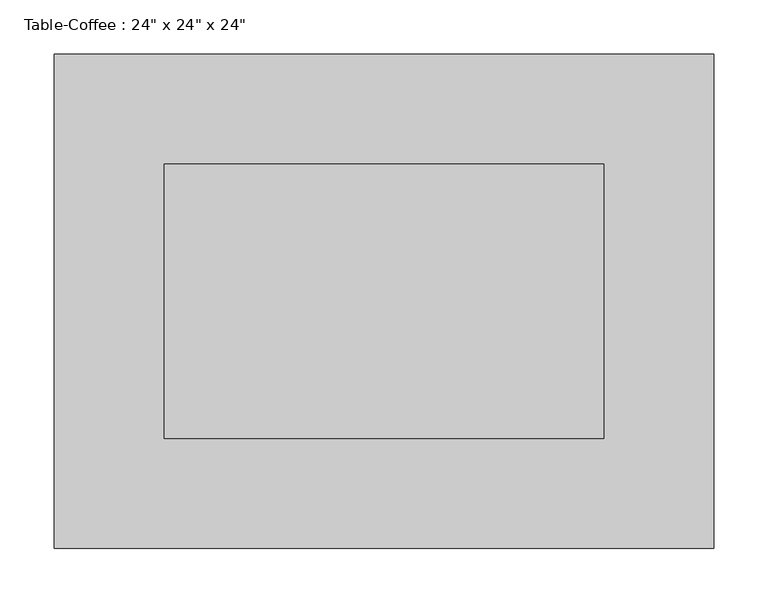
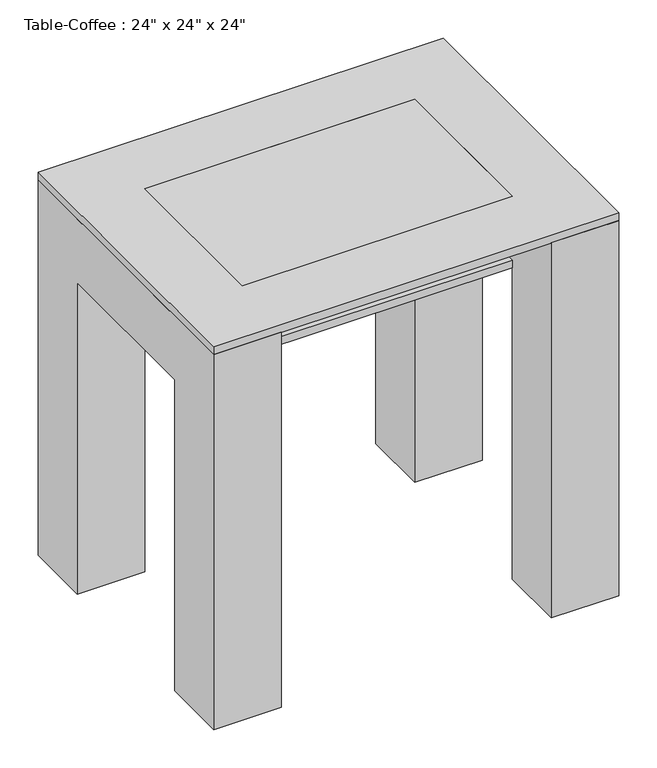
"""IFC4 building model written with IfcOpenShell, lengths in millimetres: furniture geometry."""

from ifc_helpers import new_model, si_unit, frame, origin, place, context, project, spatial, polyline, outline, extrude, source, transform, mapped, element, save


def furniture_7122704d(model_context):
    return source(origin(), model_context, "Body", "SweptSolid", [
        extrude(outline(polyline([(221.4657667, 222.2110778), (221.4657667, -31.7889222), (-184.9342333, -31.7889222), (-184.9342333, 222.2110778), (221.4657667, 222.2110778)])), frame((0.0, 0.0, 495.3), z_axis=(0.0, 0.0, 1.0), x_axis=(1.0, 0.0, 0.0)), (0.0, 0.0, 1.0), 12.7),
        extrude(outline(polyline([(323.8110778, 0.0), (222.2110778, 0.0), (222.2110778, 495.3), (-31.7889222, 495.3), (-31.7889222, 0.0), (-133.3889222, 0.0), (-133.3889222, 596.9), (323.8110778, 596.9), (323.8110778, 0.0)])), frame((221.4657667, 0.0, 0.0), z_axis=(1.0, 0.0, 0.0), x_axis=(0.0, 1.0, 0.0)), (0.0, 0.0, 1.0), 101.6),
        extrude(outline(polyline([(323.8110778, 596.9), (323.8110778, 0.0), (222.2110778, 0.0), (222.2110778, 495.3), (-31.7889222, 495.3), (-31.7889222, 0.0), (-133.3889222, 0.0), (-133.3889222, 596.9), (323.8110778, 596.9)])), frame((-286.5342333, 0.0, 0.0), z_axis=(1.0, 0.0, 0.0), x_axis=(0.0, 1.0, 0.0)), (0.0, 0.0, 1.0), 101.6),
        extrude(outline(polyline([(221.4657667, 222.2110778), (221.4657667, -31.7889222), (-184.9342333, -31.7889222), (-184.9342333, 222.2110778), (221.4657667, 222.2110778)])), frame((0.0, 0.0, 596.9), z_axis=(0.0, 0.0, 1.0), x_axis=(1.0, 0.0, 0.0)), (0.0, 0.0, 1.0), 12.7),
        extrude(outline(polyline([(323.0657667, 323.8110778), (323.0657667, -133.3889222), (-286.5342333, -133.3889222), (-286.5342333, 323.8110778), (323.0657667, 323.8110778)]), holes=[polyline([(221.4657667, 222.2110778), (-184.9342333, 222.2110778), (-184.9342333, -31.7889222), (221.4657667, -31.7889222), (221.4657667, 222.2110778)])]), frame((0.0, 0.0, 596.9), z_axis=(0.0, 0.0, 1.0), x_axis=(1.0, 0.0, 0.0)), (0.0, 0.0, 1.0), 12.7),
    ])


if __name__ == "__main__":
    model = new_model("IFC4")
    model_context = context("Model", 3, world=origin())
    ifc_project = project(units=[si_unit("LENGTHUNIT", "METRE", prefix="MILLI")], contexts=[model_context])
    site = spatial("IfcSite", under=ifc_project)
    building = spatial("IfcBuilding", under=site)
    placement = place(None, origin())
    furniture_shape = furniture_7122704d(model_context)
    element("IfcFurniture", 1, ObjectType="Table-Coffee : 24\" x 24\" x 24\"", at=placement, inside=building, context=model_context, shape_type="MappedRepresentation", body=[
        mapped(furniture_shape, transform((0.0, 0.0, 0.0), x_axis=(1.0, 0.0, 0.0), y_axis=(0.0, 1.0, 0.0), z_axis=(0.0, 0.0, 1.0))),
    ])
    save(model, "model.ifc")

# Revit data of these elements
# Type "Table-Coffee : 24\" x 24\" x 24\""
#   Assembly Code = "E2020200"
#   Height = 2' - 0"
#   Length = 2' - 0"
#   Width = 1' - 6"
#   Top Material = none
#   Frame Material = none
#   Default Elevation = 0
# Element 1 (IfcFurniture, "Table-Coffee : 24\" x 24\" x 24\"")
#   Materials on its faces: "Glass - Clear, Grey"
# Materials
#   "Glass - Clear, Grey": class "Glass", colour RGB 252 255 255, transparency 0.64
